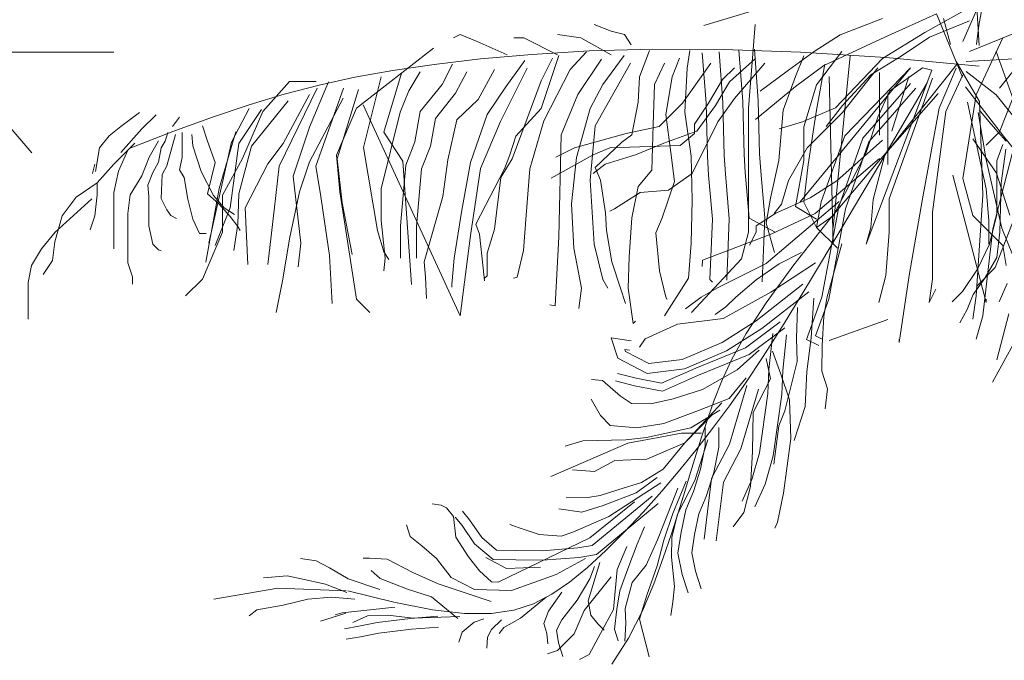
# Model space of a CAD drawing. Units: millimetres. Extents: x 595116 to 630915, y 909473 to 920225.
# Tile 20 of 134: x 629595.85 to 629606.56, y 919164.94 to 919171.91. Entities that reach past the tile are written whole.
import ezdxf

# ---------------------------------------------------------------- set-up
doc = ezdxf.new("R2010")
doc.units = ezdxf.units.MM
doc.layers.add('Dimension', color=3, linetype='Continuous', lineweight=18)
doc.layers.add('L-PLNT', color=85, linetype='Continuous', lineweight=13)
doc.styles.get("Standard").update_dxf_attribs({"font": 'arial.ttf'})
doc.dimstyles.new('ISO-25', dxfattribs={"dimtxt": 9, "dimasz": 6, "dimexe": 1.25, "dimexo": 0.625, "dimtad": 1, "dimlunit": 4, "dimtxsty": 'Standard', "dimcen": 2.5, "dimadec": 0, "dimazin": 0, "dimtfac": 1, "dimtmove": 0, "dimatfit": 3, "dimfxl": 1, "dimarcsym": 0})

# ---------------------------------------------------------------- blocks, each defined once
blk = doc.blocks.new('A$C143125F4')
for p, q in [((4.4749, 1.5142), (4.6718, 1.5142)), ((4.5077, 1.4963), (4.5843, 1.4067))]:
    blk.add_line(p, q)
blk = doc.blocks.new('A$C4FB75ABC')
for p, q in [((2.1827, 2.4393), (1.9579, 2.3712)), ((2.7686, 2.4461), (2.755, 2.3712)), ((2.4825, 2.3372), (2.6324, 2.4053)), ((2.7073, 2.4121), (2.5983, 2.3508)), ((2.6324, 2.4053), (2.7073, 2.2214)), ((2.7083, 2.3255), (2.7471, 2.4129)), ((2.7559, 2.3132), (2.7489, 2.4244)), ((1.6891, 2.3546), (1.6405, 2.3741)), ((2.1065, 2.3741), (2.087, 2.1315)), ((2.353, 2.344), (2.4757, 2.3917)), ((2.7277, 2.3849), (2.6119, 2.3372)), ((2.6732, 2.3168), (2.6528, 2.3917)), ((2.755, 2.3712), (2.7482, 2.3168)), ((1.2522, 2.3449), (1.2328, 2.3352)), ((1.3008, 2.3255), (1.2522, 2.3449)), ((1.6017, 2.3352), (1.5337, 2.3449)), ((1.7279, 2.3449), (1.6891, 2.3546)), ((1.7473, 2.3158), (1.7279, 2.3449)), ((2.2781, 2.2963), (2.353, 2.344)), ((2.5983, 2.3508), (2.4757, 2.2759)), ((2.7277, 2.2964), (2.8733, 2.3546)), ((1.3881, 2.2867), (1.3008, 2.3255)), ((1.4367, 2.3352), (1.4075, 2.3352)), ((1.5337, 2.2867), (1.4367, 2.3352)), ((1.6891, 2.2867), (1.6017, 2.3352)), ((2.3054, 2.2555), (2.4825, 2.3372)), ((2.6119, 2.3372), (2.5302, 2.2827)), ((2.8248, 2.3352), (2.7471, 2.1703)), ((1.1746, 2.3061), (0.9513, 2.1315)), ((1.4598, 2.2878), (1.3106, 2.2744)), ((1.6258, 2.2976), (1.4598, 2.2878)), ((1.5376, 2.2844), (1.4866, 2.1313)), ((1.6179, 2.2954), (1.5705, 2.2443)), ((1.8099, 2.3026), (1.6258, 2.2976)), ((1.7274, 2.2844), (1.6654, 2.2006)), ((1.8004, 2.299), (1.7712, 2.2224)), ((2.0136, 2.3019), (1.8099, 2.3026)), ((1.9171, 2.299), (1.9098, 2.248)), ((1.9536, 2.2917), (1.9646, 2.1459)), ((2.0023, 2.2954), (2.0134, 2.1483)), ((2.2382, 2.2942), (2.0136, 2.3019)), ((2.0597, 2.2997), (2.0708, 2.1511)), ((2.1047, 2.3031), (2.1159, 2.1533)), ((2.2032, 2.2419), (2.2781, 2.2963)), ((2.2482, 2.2839), (2.2239, 2.2232)), ((2.4852, 2.2785), (2.2382, 2.2942)), ((2.3575, 2.296), (2.2846, 2.199)), ((2.3818, 2.2839), (2.3332, 1.7863)), ((2.718, 2.2673), (3.0675, 2.2867)), ((2.8054, 2.2964), (2.8539, 2.1606)), ((1.1767, 2.2586), (1.0564, 2.241)), ((1.3106, 2.2744), (1.1767, 2.2586)), ((1.23, 2.2589), (1.1992, 2.2008)), ((1.4391, 2.2699), (1.3844, 2.1933)), ((1.5194, 2.2771), (1.4866, 2.2115)), ((1.6617, 2.2735), (1.5924, 2.1714)), ((1.7456, 2.2626), (1.6435, 2.0802)), ((1.8442, 2.2626), (1.815, 2.2006)), ((1.8879, 2.2771), (1.8661, 2.2224)), ((1.9783, 2.2623), (1.8966, 2.1465)), ((2.1078, 2.2759), (2.0328, 2.2078)), ((2.135, 2.2623), (2.0465, 2.1602)), ((2.2236, 2.1942), (2.3054, 2.2555)), ((2.3089, 2.2596), (2.2846, 2.1261)), ((2.4757, 2.2759), (2.3394, 2.1329)), ((2.5302, 2.2827), (2.4416, 2.2282)), ((2.6937, 2.2623), (2.4825, 1.9967)), ((2.7559, 2.2536), (2.4852, 2.2785)), ((2.6889, 2.2673), (2.7568, 2.1509)), ((1.0564, 2.241), (0.9464, 2.2213)), ((1.0815, 2.2334), (1.0304, 2.062)), ((1.1363, 2.237), (1.1034, 2.1823)), ((1.2713, 2.237), (1.2384, 2.175)), ((1.3515, 2.2443), (1.3041, 2.1568)), ((1.4464, 2.2479), (1.3687, 2.0927)), ((1.5705, 2.2443), (1.4939, 2.0948)), ((1.9098, 2.248), (1.9025, 2.1203)), ((2.0124, 2.2146), (2.0465, 2.2487)), ((2.1214, 2.1806), (2.2032, 2.2419)), ((2.5574, 2.2487), (2.2372, 1.8605)), ((2.462, 2.2487), (2.3599, 2.1193)), ((2.4416, 2.2282), (2.3599, 2.1397)), ((2.3667, 2.0512), (2.5574, 2.2487)), ((2.428, 1.738), (2.6187, 2.2419)), ((2.4668, 2.2354), (2.4668, 2.0533)), ((2.5915, 2.2487), (2.4961, 2.1806)), ((2.6187, 2.2419), (2.5915, 2.2487)), ((2.6889, 2.2479), (2.6404, 2.1315)), ((2.7083, 2.2285), (2.6598, 2.1218)), ((2.718, 2.2382), (2.8054, 2.1703)), ((2.8151, 2.1897), (2.8539, 2.2382)), ((0.7572, 2.2091), (0.6795, 2.1218)), ((0.8429, 2.1986), (0.7422, 2.1723)), ((0.8348, 2.2091), (0.7572, 2.2091)), ((0.8699, 2.2079), (0.8151, 2.0766)), ((0.9464, 2.2213), (0.8429, 2.1986)), ((1.0231, 2.2224), (0.972, 2.0182)), ((1.1992, 2.2008), (1.1362, 2.1221)), ((1.4866, 2.2115), (1.4464, 2.1021)), ((1.6654, 2.2006), (1.6289, 2.1313)), ((1.7712, 2.2224), (1.7675, 2.1495)), ((1.815, 2.2006), (1.8113, 2.0838)), ((1.8661, 2.2224), (1.8478, 2.113)), ((1.9715, 2.1465), (2.0124, 2.2146)), ((2.0328, 2.2078), (1.992, 2.1397)), ((2.2239, 2.2232), (2.1875, 2.1261)), ((2.2846, 2.199), (2.2482, 2.0776)), ((2.3211, 2.2232), (2.3332, 1.7378)), ((2.5572, 2.203), (2.4187, 2.0449)), ((2.6056, 2.2048), (2.4676, 1.9701)), ((2.6209, 2.2188), (2.4948, 1.8695)), ((2.5518, 2.2232), (2.5032, 2.0655)), ((0.7422, 2.1723), (0.6405, 2.1416)), ((0.837, 2.1896), (0.7276, 1.9635)), ((0.8151, 2.1714), (0.7385, 2.0291)), ((0.9137, 2.1896), (0.8334, 1.9635)), ((0.9575, 2.186), (0.8954, 1.9854)), ((1.1034, 2.1823), (1.0779, 2.1203)), ((1.2384, 2.175), (1.18, 2.1021)), ((1.3844, 2.1933), (1.3297, 2.113)), ((1.5924, 2.1714), (1.5449, 2.0547)), ((2.1078, 2.0989), (2.2236, 2.1942)), ((2.5724, 2.1897), (2.4365, 2.0345)), ((2.4961, 2.1806), (2.462, 2.1057)), ((2.6368, 2.1742), (2.4628, 1.9766)), ((2.4911, 2.1747), (2.4911, 1.9684)), ((2.7471, 2.1703), (2.7083, 1.9277)), ((2.7162, 2.1941), (2.8268, 2.0511)), ((2.8054, 2.1703), (2.883, 2.0733)), ((0.6405, 2.1416), (0.5342, 2.1057)), ((0.7531, 2.1531), (0.6473, 2.0218)), ((0.9125, 2.1606), (0.8154, 1.9763)), ((1.2522, 1.53), (0.9707, 2.1412)), ((1.3041, 2.1568), (1.2421, 2.0984)), ((1.7675, 2.1495), (1.7493, 2.0547)), ((1.8966, 2.1465), (1.8285, 2.0784)), ((1.9306, 2.0852), (1.9715, 2.1465)), ((1.9646, 2.1459), (1.9682, 1.9927)), ((2.0465, 2.1602), (1.9988, 2.0921)), ((2.0134, 2.1483), (2.017, 1.9949)), ((2.0708, 2.1511), (2.0745, 1.9975)), ((2.1159, 2.1533), (2.1196, 1.9995)), ((2.7225, 2.1495), (2.753, 2.0047)), ((2.7568, 2.1509), (2.7666, 1.8792)), ((2.8927, 2.1606), (2.7957, 1.7822)), ((2.8539, 2.1606), (2.8151, 2.0636)), ((0.2683, 2.0784), (0.3228, 2.1193)), ((0.3296, 2.0716), (0.3705, 2.1125)), ((0.64, 2.1313), (0.5889, 2.0328)), ((0.6765, 2.1276), (0.6108, 2.0291)), ((0.6795, 2.1218), (0.6213, 1.986)), ((0.9513, 2.1315), (0.8931, 1.9957)), ((1.0779, 2.1203), (1.0231, 1.8978)), ((1.1362, 2.1221), (1.1203, 2.0346)), ((1.3297, 2.113), (1.2822, 1.9744)), ((1.4866, 2.1313), (1.4136, 2.051)), ((1.6289, 2.1313), (1.5887, 1.989)), ((1.8478, 2.113), (1.8624, 2.0036)), ((1.9025, 2.1203), (1.9208, 1.9927)), ((1.992, 2.1397), (1.9375, 2.0648)), ((2.087, 2.1315), (2.087, 1.7725)), ((2.1875, 2.1261), (2.1754, 1.9805)), ((2.3394, 2.1329), (2.244, 2.0921)), ((2.3599, 2.1193), (2.2577, 2.0172)), ((2.2846, 2.1261), (2.2604, 1.9684)), ((2.3599, 2.1397), (2.3122, 2.0784)), ((2.6404, 2.1315), (2.5918, 1.8695)), ((2.6598, 2.1218), (2.6209, 1.8307)), ((2.753, 2.119), (2.7759, 1.9818)), ((2.7555, 2.1274), (2.7844, 2.0931)), ((0.4182, 2.0784), (0.4386, 2.1057)), ((0.5342, 2.1057), (0.4195, 2.0639)), ((1.18, 2.1021), (1.1654, 2.0218)), ((1.2421, 2.0984), (1.2165, 1.9817)), ((1.3687, 2.0927), (1.3105, 1.9569)), ((1.4464, 2.1021), (1.4026, 1.9854)), ((1.4939, 2.0948), (1.4537, 1.9562)), ((1.8113, 2.0838), (1.8077, 1.9526)), ((1.9988, 2.0921), (1.9238, 1.9422)), ((1.9306, 2.058), (1.9306, 2.0852)), ((2.244, 2.0921), (2.1759, 2.0716)), ((2.462, 2.1057), (2.428, 2.0035)), ((2.7844, 2.0931), (2.8104, 2.0628)), ((0.2342, 2.0512), (0.2683, 2.0784)), ((0.2683, 2.0035), (0.3296, 2.0716)), ((0.4195, 2.0639), (0.2927, 2.0154)), ((0.4049, 2.0609), (0.3966, 2.0361)), ((0.427, 2.0554), (0.4021, 1.9643)), ((0.4463, 2.0609), (0.4463, 1.9892)), ((0.4739, 2.0554), (0.4767, 2.0223)), ((0.505, 2.0802), (0.5196, 2.0364)), ((0.6018, 2.0636), (0.5533, 1.8986)), ((0.8151, 2.0766), (0.7677, 1.9343)), ((1.0304, 2.062), (1.0852, 1.9781)), ((1.5449, 2.0547), (1.5376, 1.7593)), ((1.7331, 2.058), (1.5832, 2.0172)), ((1.6435, 2.0802), (1.6289, 1.9234)), ((1.7493, 2.0547), (1.7201, 2.0328)), ((1.8285, 2.0784), (1.7331, 2.058)), ((1.9375, 2.0648), (1.8421, 2.0308)), ((1.8898, 2.024), (1.9306, 2.058)), ((2.2482, 2.0776), (2.2482, 1.9805)), ((2.8151, 2.0636), (2.7763, 2.0248)), ((2.8104, 2.0628), (2.8339, 2.0359)), ((0.207, 2.0172), (0.2342, 2.0512)), ((0.3092, 2.0308), (0.2479, 1.9695)), ((0.3773, 2.0376), (0.3501, 1.9899)), ((0.3966, 2.0361), (0.3855, 2.0168)), ((0.5196, 2.0364), (0.5415, 1.9744)), ((0.5889, 2.0328), (0.5232, 1.741)), ((0.6108, 2.0291), (0.5853, 1.8431)), ((0.7385, 2.0291), (0.6947, 1.9708)), ((1.1203, 2.0346), (1.0939, 1.9669)), ((1.4136, 2.051), (1.3953, 1.9963)), ((1.7201, 2.0328), (1.6435, 1.9598)), ((1.8421, 2.0308), (1.7603, 1.9967)), ((2.2985, 1.8605), (2.3667, 2.0512)), ((2.4756, 2.0387), (2.3438, 1.9217)), ((2.4187, 2.0449), (2.3489, 1.8456)), ((2.4365, 2.0345), (2.3686, 1.8404)), ((2.7378, 2.0428), (2.8064, 1.9437)), ((2.8244, 2.0263), (2.8071, 1.979)), ((2.8268, 2.0511), (2.9214, 1.9326)), ((0.195, 1.9478), (0.207, 2.0172)), ((0.2887, 2.0103), (0.2615, 1.9491)), ((0.3855, 2.0168), (0.3773, 1.9754)), ((0.4767, 2.0223), (0.5015, 1.9478)), ((0.6473, 2.0218), (0.6108, 1.8833)), ((0.972, 2.0182), (1.0122, 1.7775)), ((1.1654, 2.0218), (1.1399, 1.9562)), ((1.5832, 2.0172), (1.5287, 1.9899)), ((1.6377, 1.9967), (1.6854, 2.0172)), ((1.6854, 2.0172), (1.8898, 2.024)), ((1.8624, 2.0036), (1.8734, 1.9197)), ((2.0745, 1.9975), (2.0779, 1.946)), ((2.1196, 1.9995), (2.1229, 1.9495)), ((2.2577, 2.0172), (2.2032, 1.9218)), ((2.428, 2.0035), (2.3871, 1.9218)), ((2.753, 2.0047), (2.7759, 1.898)), ((2.833, 2.0134), (2.8201, 1.9144)), ((0.1865, 1.9422), (0.1934, 1.9695)), ((0.2479, 1.9695), (0.2002, 1.915)), ((0.3501, 1.9899), (0.3296, 1.9354)), ((0.3773, 1.9754), (0.3607, 1.945)), ((0.4463, 1.9892), (0.438, 1.9533)), ((0.5415, 1.9744), (0.5196, 1.8833)), ((0.6213, 1.986), (0.563, 1.8792)), ((0.6947, 1.9708), (0.629, 1.8431)), ((0.8154, 1.9763), (0.7863, 1.8889)), ((0.8931, 1.9957), (0.9028, 1.8889)), ((0.8954, 1.9854), (0.91, 1.8577)), ((1.0852, 1.9781), (1.1107, 1.6207)), ((1.2165, 1.9817), (1.2019, 1.876)), ((1.2822, 1.9744), (1.2567, 1.8358)), ((1.4026, 1.9854), (1.3698, 1.9307)), ((1.3953, 1.9963), (1.3807, 1.9562)), ((1.5151, 1.9286), (1.6377, 1.9967)), ((1.5887, 1.989), (1.5741, 1.8541)), ((1.6718, 1.9695), (1.6377, 1.9422)), ((1.7603, 1.9967), (1.6718, 1.9695)), ((1.9208, 1.9927), (1.9244, 1.865)), ((1.9682, 1.9927), (1.9719, 1.938)), ((2.017, 1.9949), (2.0206, 1.9417)), ((2.1754, 1.9805), (2.1511, 1.8713)), ((2.2482, 1.9805), (2.2239, 1.847)), ((2.4673, 1.986), (2.2802, 1.8264)), ((2.4628, 1.9766), (2.3249, 1.8127)), ((2.4676, 1.9701), (2.3552, 1.7802)), ((2.4825, 1.9967), (2.4484, 1.8673)), ((2.7759, 1.9818), (2.8217, 1.7836)), ((2.8071, 1.979), (2.8071, 1.9015)), ((0.2615, 1.9491), (0.2479, 1.8878)), ((0.3607, 1.945), (0.3469, 1.9091)), ((0.4021, 1.9643), (0.3883, 1.9395)), ((0.438, 1.9533), (0.4518, 1.9312)), ((0.5015, 1.9478), (0.5374, 1.8788)), ((0.7276, 1.9635), (0.713, 1.8358)), ((0.8334, 1.9635), (0.848, 1.876)), ((1.0939, 1.9669), (1.0786, 1.7905)), ((1.1399, 1.9562), (1.1253, 1.7884)), ((1.3105, 1.9569), (1.2814, 1.7628)), ((1.3807, 1.9562), (1.2968, 1.7957)), ((1.4537, 1.9562), (1.4428, 1.8213)), ((1.6435, 1.9598), (1.6581, 1.9234)), ((1.8077, 1.9526), (1.7675, 1.9051)), ((1.9238, 1.9422), (1.8557, 1.8946)), ((2.0206, 1.9417), (2.0317, 1.8114)), ((2.0779, 1.946), (2.0893, 1.8127)), ((2.1229, 1.9495), (2.1345, 1.8136)), ((2.2604, 1.9684), (2.2482, 1.8591)), ((2.8064, 1.9437), (2.8446, 1.8217)), ((0.2002, 1.915), (0.1389, 1.8742)), ((0.2002, 1.915), (0.2002, 1.881)), ((0.3296, 1.9354), (0.2956, 1.881)), ((0.3883, 1.9395), (0.3855, 1.8705)), ((0.4518, 1.9312), (0.4629, 1.8677)), ((0.7677, 1.9343), (0.7896, 1.741)), ((1.3698, 1.9307), (1.3515, 1.7811)), ((1.6289, 1.9234), (1.6398, 1.7374)), ((1.6581, 1.9234), (1.6727, 1.8285)), ((1.8734, 1.9197), (1.8369, 1.814)), ((1.9719, 1.938), (1.9828, 1.8103)), ((2.2032, 1.9218), (2.1827, 1.8537)), ((2.3438, 1.9217), (2.2657, 1.8718)), ((2.3871, 1.9218), (2.3326, 1.8197)), ((2.6792, 1.9375), (2.7763, 1.5688)), ((2.7083, 1.9277), (2.7374, 1.821)), ((2.8201, 1.9144), (2.8158, 1.7724)), ((0.2479, 1.8878), (0.2479, 1.8061)), ((0.3469, 1.9091), (0.3497, 1.876)), ((0.5533, 1.8986), (0.5339, 1.7919)), ((0.7863, 1.8889), (0.7572, 1.7531)), ((0.9028, 1.8889), (0.9513, 1.5785)), ((1.0231, 1.8978), (1.0231, 1.8067)), ((1.7739, 1.8878), (1.699, 1.8401)), ((1.7675, 1.9051), (1.7493, 1.814)), ((1.8557, 1.8946), (1.7739, 1.8878)), ((2.7759, 1.898), (2.7836, 1.8065)), ((2.8071, 1.9015), (2.8071, 1.8241)), ((0.1844, 1.8695), (0.0777, 1.7725)), ((0.1389, 1.8742), (0.098, 1.8197)), ((0.2002, 1.881), (0.1934, 1.8197)), ((0.2956, 1.881), (0.2887, 1.8265)), ((0.3497, 1.876), (0.3497, 1.8512)), ((0.3855, 1.8705), (0.4021, 1.8374)), ((0.4629, 1.8677), (0.4767, 1.8098)), ((0.5196, 1.8833), (0.5524, 1.8541)), ((0.5374, 1.8788), (0.5678, 1.8429)), ((0.563, 1.8792), (0.563, 1.7725)), ((0.6108, 1.8833), (0.6072, 1.7957)), ((0.848, 1.876), (0.8735, 1.7045)), ((0.91, 1.8577), (0.9392, 1.7082)), ((1.2019, 1.876), (1.1472, 1.6863)), ((1.9244, 1.865), (1.9208, 1.741)), ((2.3505, 1.8613), (2.1386, 1.6813)), ((2.1511, 1.8713), (2.1389, 1.7985)), ((2.2657, 1.8718), (2.167, 1.8279)), ((2.2482, 1.8591), (2.2846, 1.7863)), ((2.2849, 1.7856), (2.2985, 1.8605)), ((2.4484, 1.8673), (2.4416, 1.7856)), ((2.4948, 1.8695), (2.4948, 1.7725)), ((2.5918, 1.8695), (2.553, 1.6464)), ((2.7666, 1.8792), (2.7471, 1.5882)), ((0.2887, 1.8265), (0.2887, 1.7516)), ((0.3497, 1.8512), (0.3497, 1.7904)), ((0.4021, 1.8374), (0.4132, 1.8208)), ((0.5853, 1.8431), (0.5415, 1.7337)), ((0.5524, 1.8541), (0.5853, 1.8176)), ((0.5678, 1.8429), (0.5982, 1.8236)), ((0.629, 1.8431), (0.6363, 1.679)), ((0.713, 1.8358), (0.6984, 1.7118)), ((1.2567, 1.8358), (1.2348, 1.6973)), ((1.5741, 1.8541), (1.5814, 1.7264)), ((1.6727, 1.8285), (1.6763, 1.7775)), ((1.699, 1.8401), (1.6854, 1.8333)), ((2.167, 1.8279), (2.1099, 1.791)), ((2.2802, 1.8264), (2.1549, 1.7678)), ((2.1827, 1.8537), (2.1623, 1.8265)), ((2.2239, 1.847), (2.2846, 1.8106)), ((2.3489, 1.8456), (2.3004, 1.5838)), ((2.3686, 1.8404), (2.32, 1.5785)), ((2.6209, 1.8307), (2.6209, 1.6367)), ((2.8708, 1.8469), (2.8027, 1.6699)), ((0.098, 1.8197), (0.0775, 1.7448)), ((0.1934, 1.8197), (0.1797, 1.7788)), ((0.2479, 1.8061), (0.2479, 1.7448)), ((0.4132, 1.8208), (0.4297, 1.8125)), ((0.4767, 1.8098), (0.496, 1.7684)), ((0.5853, 1.8176), (0.6072, 1.7884)), ((1.0231, 1.8067), (1.0341, 1.6973)), ((1.4428, 1.8213), (1.4355, 1.7191)), ((1.7493, 1.814), (1.742, 1.7009)), ((1.8369, 1.814), (1.8186, 1.7702)), ((1.9828, 1.8103), (1.9755, 1.6352)), ((2.0317, 1.8114), (2.0243, 1.6332)), ((2.0893, 1.8127), (2.1647, 1.7725)), ((2.1345, 1.8136), (2.1268, 1.6289)), ((2.1389, 1.7985), (2.1632, 1.7135)), ((2.3249, 1.8127), (2.2184, 1.678)), ((2.3326, 1.8197), (2.2849, 1.7856)), ((2.7374, 1.821), (2.8248, 1.7337)), ((2.7836, 1.8065), (2.7836, 1.7379)), ((2.8071, 1.8241), (2.7856, 1.738)), ((0.0777, 1.7725), (0.0388, 1.724)), ((0.3497, 1.7904), (0.3607, 1.738)), ((0.563, 1.7725), (0.5048, 1.6367)), ((0.5339, 1.7919), (0.5145, 1.6852)), ((0.6072, 1.7957), (0.5962, 1.7191)), ((0.6072, 1.7884), (0.6144, 1.7775)), ((1.0122, 1.7775), (1.0304, 1.7155)), ((1.0786, 1.7905), (1.0786, 1.6973)), ((1.1253, 1.7884), (1.1253, 1.7665)), ((1.2968, 1.7957), (1.3078, 1.7665)), ((1.3515, 1.7811), (1.3297, 1.7118)), ((1.6763, 1.7775), (1.6909, 1.6863)), ((1.8186, 1.7702), (1.8296, 1.6608)), ((2.087, 1.7725), (2.0676, 1.6949)), ((2.1096, 1.7722), (2.0903, 1.7347)), ((2.1099, 1.791), (2.1096, 1.7722)), ((2.3552, 1.7802), (2.2641, 1.6283)), ((2.2846, 1.7863), (2.3453, 1.7256)), ((2.4416, 1.7856), (2.428, 1.738)), ((2.4948, 1.7725), (2.485, 1.6464)), ((2.7957, 1.7822), (2.7666, 1.53)), ((2.8158, 1.7724), (2.8071, 1.6993)), ((2.8217, 1.7836), (2.8522, 1.7074)), ((0.0775, 1.7448), (0.0707, 1.6903)), ((0.2479, 1.7448), (0.2479, 1.7243)), ((0.2887, 1.7516), (0.2887, 1.6835)), ((0.496, 1.7684), (0.5153, 1.7684)), ((0.7572, 1.7531), (0.7377, 1.6367)), ((0.7896, 1.741), (0.7823, 1.6717)), ((1.1253, 1.7665), (1.1253, 1.7301)), ((1.2814, 1.7628), (1.2522, 1.53)), ((1.3078, 1.7665), (1.3187, 1.6681)), ((1.5376, 1.7593), (1.5267, 1.5587)), ((1.9208, 1.741), (1.9135, 1.6389)), ((2.1549, 1.7678), (1.9538, 1.6913)), ((0.0388, 1.724), (0.0097, 1.6755)), ((0.3607, 1.738), (0.3773, 1.7214)), ((0.3773, 1.7214), (0.3855, 1.7187)), ((1.0304, 1.7155), (1.045, 1.6936)), ((1.1253, 1.7301), (1.1253, 1.6973)), ((1.4355, 1.7191), (1.4172, 1.6425)), ((1.5814, 1.7264), (1.6033, 1.6097)), ((1.6398, 1.7374), (1.6654, 1.6352)), ((2.2409, 1.7138), (2.1763, 1.6807)), ((2.3582, 1.7386), (2.3145, 1.5808)), ((2.7856, 1.738), (2.7512, 1.6648)), ((2.8248, 1.7337), (2.8345, 1.6755)), ((0.0707, 1.6903), (0.0435, 1.6494)), ((0.6984, 1.7118), (0.6947, 1.679)), ((0.8735, 1.7045), (0.8808, 1.566)), ((1.0341, 1.6973), (1.0304, 1.6608)), ((1.1472, 1.6863), (1.1509, 1.6425)), ((1.2348, 1.6973), (1.2275, 1.6207)), ((1.3297, 1.7118), (1.3297, 1.6462)), ((1.6909, 1.6863), (1.7164, 1.6097)), ((1.742, 1.7009), (1.7383, 1.6097)), ((2.0676, 1.6949), (1.922, 1.5397)), ((1.9538, 1.6913), (1.9536, 1.6725)), ((2.8071, 1.6993), (2.7727, 1.639)), ((0.0097, 1.6755), (0, 1.627)), ((0.2887, 1.6835), (0.3024, 1.6426)), ((1.3187, 1.6681), (1.3224, 1.6316)), ((1.8296, 1.6608), (1.8478, 1.5842)), ((2.1386, 1.6813), (1.998, 1.6115)), ((2.1763, 1.6807), (2.1096, 1.6345)), ((2.2184, 1.678), (2.1385, 1.568)), ((2.2819, 1.6831), (2.1525, 1.5981)), ((2.7512, 1.6648), (2.7081, 1.6003)), ((2.8027, 1.6699), (2.7482, 1.6154)), ((0, 1.627), (0, 1.5494)), ((0.3024, 1.6426), (0.3024, 1.6222)), ((0.5048, 1.6367), (0.4562, 1.5882)), ((0.7377, 1.6367), (0.7183, 1.5397)), ((1.1509, 1.6425), (1.1545, 1.5805)), ((1.3297, 1.6462), (1.3224, 1.6389)), ((1.4172, 1.6425), (1.4063, 1.6389)), ((1.6654, 1.6352), (1.68, 1.6097)), ((1.9135, 1.6389), (1.8444, 1.53)), ((1.9755, 1.6352), (1.9828, 1.628)), ((2.1096, 1.6345), (2.0504, 1.5844)), ((2.2641, 1.6283), (2.1904, 1.5079)), ((2.485, 1.6464), (2.4656, 1.5688)), ((2.553, 1.6464), (2.5239, 1.4523)), ((2.6209, 1.6367), (2.6112, 1.5688)), ((2.7727, 1.639), (2.7383, 1.5917)), ((1.2275, 1.6207), (1.2275, 1.6134)), ((1.6033, 1.6097), (1.596, 1.5514)), ((1.7164, 1.6097), (1.731, 1.566)), ((1.7383, 1.6097), (1.7529, 1.5076)), ((1.998, 1.6115), (1.9504, 1.5839)), ((2.1525, 1.5981), (2.0137, 1.5227)), ((2.2452, 1.6213), (2.1098, 1.5157)), ((2.2623, 1.5995), (2.1258, 1.493)), ((2.6112, 1.5688), (2.6307, 1.6076)), ((2.7081, 1.6003), (2.678, 1.5702)), ((2.8369, 1.6236), (2.8141, 1.5702)), ((0.9513, 1.5785), (0.9901, 1.5397)), ((1.8478, 1.5842), (1.8515, 1.5769)), ((1.9504, 1.5839), (1.9047, 1.5506)), ((2.0504, 1.5844), (2.0217, 1.5565)), ((2.3004, 1.5838), (2.256, 1.4617)), ((2.2767, 1.5813), (2.2695, 1.4664)), ((2.32, 1.5785), (2.2812, 1.4717)), ((2.3145, 1.5808), (2.3062, 1.5281)), ((2.7383, 1.5917), (2.721, 1.5486)), ((2.7471, 1.5882), (2.7374, 1.5203)), ((2.7763, 1.5688), (2.7763, 1.5785)), ((0, 1.5494), (0, 1.5203)), ((1.5267, 1.5587), (1.5121, 1.5623)), ((2.0217, 1.5565), (1.9912, 1.5343)), ((2.1385, 1.568), (2.0803, 1.4783)), ((2.2292, 1.5537), (2.2261, 1.4651)), ((2.721, 1.5486), (2.6995, 1.5099)), ((2.9148, 1.5573), (2.7942, 1.3378)), ((1.7529, 1.5076), (1.7602, 1.5149)), ((2.0137, 1.5227), (1.8814, 1.5056)), ((2.1098, 1.5157), (2.0109, 1.453)), ((2.1796, 1.5129), (2.0785, 1.437)), ((2.3062, 1.5281), (2.3013, 1.4452)), ((2.4911, 1.5193), (2.3211, 1.4586)), ((2.7666, 1.53), (2.7471, 1.462)), ((2.8416, 1.5357), (2.8071, 1.4023)), ((1.8814, 1.5056), (1.7884, 1.4636)), ((2.1258, 1.493), (2.0238, 1.4284)), ((2.1927, 1.4954), (2.0894, 1.4177)), ((2.1904, 1.5079), (2.1298, 1.4122)), ((1.7084, 1.4073), (1.6895, 1.4666)), ((1.6895, 1.4666), (1.747, 1.4576)), ((1.7884, 1.4636), (1.7711, 1.4393)), ((2.0803, 1.4783), (2.039, 1.4043)), ((2.1578, 1.4791), (2.1468, 1.3743)), ((2.1979, 1.4749), (2.187, 1.3714)), ((2.2261, 1.4651), (2.2289, 1.3972)), ((2.256, 1.4617), (2.2916, 1.4439)), ((2.2695, 1.4664), (2.2568, 1.3685)), ((2.2812, 1.4717), (2.3006, 1.462)), ((2.5239, 1.4523), (2.5239, 1.462)), ((1.7313, 1.4266), (1.7295, 1.4323)), ((1.7295, 1.4323), (1.7427, 1.4302)), ((2.0109, 1.453), (1.8951, 1.4036)), ((2.0238, 1.4284), (1.9024, 1.3766)), ((2.0785, 1.437), (1.9344, 1.3786)), ((2.1181, 1.4308), (2.055, 1.3732)), ((2.1569, 1.4277), (2.1816, 1.3609)), ((2.3013, 1.4452), (2.3002, 1.3698)), ((1.7936, 1.3632), (1.7084, 1.4073)), ((1.7987, 1.3918), (1.7313, 1.4266)), ((1.8951, 1.4036), (1.7987, 1.3918)), ((2.0894, 1.4177), (1.9429, 1.3584)), ((2.039, 1.4043), (2.0098, 1.3416)), ((2.1298, 1.4122), (2.0784, 1.3347)), ((2.1385, 1.406), (2.1509, 1.3473)), ((1.9024, 1.3766), (1.7936, 1.3632)), ((1.9344, 1.3786), (1.8357, 1.3347)), ((2.055, 1.3732), (1.9542, 1.3161)), ((2.1468, 1.3743), (2.1439, 1.3053)), ((2.187, 1.3714), (2.1842, 1.3016)), ((2.2289, 1.3972), (2.1929, 1.2544)), ((2.3002, 1.3698), (2.3165, 1.3187)), ((1.6641, 1.3427), (1.6321, 1.345)), ((1.7163, 1.2967), (1.6641, 1.3427)), ((1.7575, 1.3275), (1.7024, 1.3416)), ((1.7623, 1.3489), (1.7078, 1.3628)), ((1.8357, 1.3347), (1.7623, 1.3489)), ((1.9429, 1.3584), (1.8383, 1.3119)), ((2.0098, 1.3416), (1.9878, 1.2857)), ((2.0811, 1.3502), (2.0312, 1.2905)), ((2.1509, 1.3473), (2.1005, 1.25)), ((2.1816, 1.3609), (2.2062, 1.287)), ((2.2568, 1.3685), (2.2516, 1.2668)), ((1.8383, 1.3119), (1.7575, 1.3275)), ((1.9542, 1.3161), (1.869, 1.289)), ((2.0784, 1.3347), (2.0319, 1.2687)), ((2.0829, 1.3276), (2.0324, 1.158)), ((2.1165, 1.3176), (2.065, 1.1449)), ((2.3165, 1.3187), (2.31, 1.2603)), ((1.6589, 1.2409), (1.6313, 1.2885)), ((1.7481, 1.2755), (1.7163, 1.2967)), ((1.869, 1.289), (1.8046, 1.2748)), ((2.0312, 1.2905), (1.9421, 1.2559)), ((1.9878, 1.2857), (1.9691, 1.2327)), ((2.1439, 1.3053), (2.1195, 1.1332)), ((2.1842, 1.3016), (2.1591, 1.1247)), ((2.2062, 1.287), (2.2097, 1.1745)), ((1.8046, 1.2748), (1.7481, 1.2755)), ((1.9421, 1.2559), (1.8416, 1.2177)), ((2.0103, 1.2776), (1.903, 1.1622)), ((2.0043, 1.257), (1.9206, 1.2053)), ((2.0319, 1.2687), (1.9864, 1.2075)), ((2.2516, 1.2668), (2.22, 1.1691)), ((1.6868, 1.2123), (1.6589, 1.2409)), ((1.9834, 1.244), (1.903, 1.1622)), ((1.9691, 1.2327), (1.952, 1.1808)), ((2.1005, 1.25), (2.0989, 1.1369)), ((2.1929, 1.2544), (2.1754, 1.2112)), ((1.7641, 1.2056), (1.6868, 1.2123)), ((1.8416, 1.2177), (1.7641, 1.2056)), ((1.9206, 1.2053), (1.792, 1.1769)), ((1.9864, 1.2075), (1.9386, 1.1458)), ((1.9621, 1.2066), (1.9614, 1.1536)), ((2.0017, 1.2061), (2.001, 1.1495)), ((2.1754, 1.2112), (2.1606, 1.1002)), ((1.7315, 1.1702), (1.607, 1.1681)), ((1.792, 1.1769), (1.7315, 1.1702)), ((1.7376, 1.1613), (1.8929, 1.1904)), ((1.8929, 1.1904), (1.9511, 1.1904)), ((1.9692, 1.1707), (1.9317, 1.0524)), ((1.952, 1.1808), (1.9358, 1.129)), ((2.2097, 1.1745), (2.1886, 1.0162)), ((1.5143, 1.0642), (1.7376, 1.1613)), ((1.607, 1.1681), (1.5558, 1.1518)), ((1.903, 1.1622), (1.793, 1.1147)), ((1.903, 1.1622), (1.8397, 1.0857)), ((1.9386, 1.1458), (1.8882, 1.0835)), ((1.9614, 1.1536), (1.9482, 1.0859)), ((2.0324, 1.158), (1.9806, 1.0581)), ((2.001, 1.1495), (1.9867, 1.0762)), ((2.065, 1.1449), (2.0146, 1.0475)), ((1.793, 1.1147), (1.7005, 1.1103)), ((1.9358, 1.129), (1.9198, 1.076)), ((2.0989, 1.1369), (2.0937, 1.0351)), ((2.1195, 1.1332), (2.0972, 1.056)), ((2.1591, 1.1247), (2.1353, 1.0421)), ((1.7005, 1.1103), (1.6416, 1.079)), ((1.8397, 1.0857), (1.7769, 1.047)), ((1.9482, 1.0859), (1.9278, 1.0204)), ((1.6416, 1.079), (1.5775, 1.0837)), ((1.8224, 1.0615), (1.7614, 1.017)), ((1.8882, 1.0835), (1.8359, 1.0215)), ((1.9198, 1.076), (1.903, 1.0206)), ((1.9806, 1.0581), (1.9586, 0.8825)), ((1.9867, 1.0762), (1.965, 1.0067)), ((2.0972, 1.056), (2.0692, 0.9929)), ((1.8335, 1.0462), (1.6831, 0.9483)), ((1.7769, 1.047), (1.7087, 1.0253)), ((1.8823, 1.0305), (1.8549, 0.9592)), ((1.9071, 1.0509), (1.8681, 0.9571)), ((1.9317, 1.0524), (1.8813, 0.9551)), ((2.0146, 1.0475), (2.004, 0.9628)), ((2.0937, 1.0351), (2.0738, 0.96)), ((2.1353, 1.0421), (2.1061, 0.9765)), ((1.6216, 1.0039), (1.5594, 1.0028)), ((1.6576, 1.009), (1.6216, 1.0039)), ((1.8084, 1.007), (1.6348, 0.8642)), ((1.7087, 1.0253), (1.6576, 1.009)), ((1.7614, 1.017), (1.6666, 0.9806)), ((1.8359, 1.0215), (1.7823, 0.9612)), ((1.903, 1.0206), (1.8847, 0.9618)), ((1.9278, 1.0204), (1.9055, 0.9679)), ((1.965, 1.0067), (1.9435, 0.9561)), ((2.1886, 1.0162), (2.171, 0.9318)), ((1.1969, 0.9814), (1.1705, 0.9855)), ((1.2119, 0.9737), (1.1969, 0.9814)), ((1.2323, 0.9489), (1.2119, 0.9737)), ((1.6041, 0.9607), (1.5382, 0.9711)), ((1.6666, 0.9806), (1.6041, 0.9607)), ((1.7573, 0.9907), (1.6276, 0.8869)), ((1.8259, 0.9857), (1.6466, 0.8382)), ((1.239, 0.8884), (1.2323, 0.9489)), ((1.2572, 0.9222), (1.2376, 0.9461)), ((1.2793, 0.9388), (1.2589, 0.9636)), ((1.6831, 0.9483), (1.5787, 0.9026)), ((1.7823, 0.9612), (1.7281, 0.9036)), ((1.8549, 0.9592), (1.8236, 0.8804)), ((1.8681, 0.9571), (1.8425, 0.8802)), ((1.8847, 0.9618), (1.8642, 0.8983)), ((1.8813, 0.9551), (1.8652, 0.8874)), ((1.9055, 0.9679), (1.8924, 0.9029)), ((1.9435, 0.9561), (1.9314, 0.8959)), ((2.004, 0.9628), (1.9934, 0.8781)), ((2.0738, 0.96), (2.043, 0.9189)), ((1.107, 0.8902), (1.0961, 0.9243)), ((1.2938, 0.8688), (1.2572, 0.9222)), ((1.3144, 0.8874), (1.2793, 0.9388)), ((1.4036, 0.922), (1.3961, 0.9259)), ((1.4317, 0.9122), (1.4036, 0.922)), ((1.7864, 0.9186), (1.765, 0.868)), ((2.171, 0.9318), (2.164, 0.9142)), ((1.1405, 0.8634), (1.107, 0.8902)), ((1.2759, 0.8314), (1.239, 0.8884)), ((1.3573, 0.851), (1.3144, 0.8874)), ((1.6276, 0.8869), (1.3617, 0.7585)), ((1.4805, 0.8964), (1.4317, 0.9122)), ((1.5446, 0.8918), (1.4805, 0.8964)), ((1.5787, 0.9026), (1.5446, 0.8918)), ((1.7281, 0.9036), (1.6739, 0.8498)), ((1.8642, 0.8983), (1.8405, 0.829)), ((1.8652, 0.8874), (1.8644, 0.8308)), ((1.8924, 0.9029), (1.8829, 0.8424)), ((1.9314, 0.8959), (1.9231, 0.8432)), ((1.1834, 0.827), (1.1405, 0.8634)), ((1.347, 0.8236), (1.2938, 0.8688)), ((1.5932, 0.8572), (1.4893, 0.8492)), ((1.6348, 0.8642), (1.5932, 0.8572)), ((1.7347, 0.8614), (1.7065, 0.7946)), ((1.765, 0.868), (1.7376, 0.7967)), ((1.8236, 0.8804), (1.7906, 0.8073)), ((1.8425, 0.8802), (1.8226, 0.805)), ((0.9891, 0.8277), (0.9703, 0.828)), ((1.04, 0.8252), (0.9891, 0.8277)), ((1.3074, 0.7913), (1.2759, 0.8314)), ((1.3863, 0.7981), (1.3265, 0.8298)), ((1.4139, 0.8502), (1.3573, 0.851)), ((1.4893, 0.8492), (1.4139, 0.8502)), ((1.5965, 0.8298), (1.4902, 0.8216)), ((1.6466, 0.8382), (1.5965, 0.8298)), ((1.6739, 0.8498), (1.6204, 0.8011)), ((1.8405, 0.829), (1.8129, 0.7535)), ((1.8644, 0.8308), (1.8727, 0.7459)), ((1.8829, 0.8424), (1.8952, 0.7804)), ((1.9231, 0.8432), (1.9337, 0.7903)), ((0.8346, 0.8198), (0.7888, 0.827)), ((0.8736, 0.7996), (0.8346, 0.8198)), ((0.9273, 0.7678), (0.8736, 0.7996)), ((1.1149, 0.7864), (1.04, 0.8252)), ((1.226, 0.7717), (1.1834, 0.827)), ((1.4135, 0.8227), (1.347, 0.8236)), ((1.4848, 0.8016), (1.3863, 0.7981)), ((1.4902, 0.8216), (1.4135, 0.8227)), ((1.6154, 0.8267), (1.5299, 0.7807)), ((1.6204, 0.8011), (1.5682, 0.7585)), ((1.6567, 0.8148), (1.6231, 0.704)), ((1.6415, 0.8037), (1.6278, 0.7681)), ((1.7906, 0.8073), (1.7502, 0.757)), ((1.8226, 0.805), (1.7931, 0.7206)), ((0.7503, 0.7767), (0.6814, 0.7711)), ((0.7912, 0.768), (0.7503, 0.7767)), ((1.0204, 0.7689), (0.9943, 0.7918)), ((1.188, 0.7534), (1.1149, 0.7864)), ((1.2935, 0.7368), (1.226, 0.7717)), ((1.3428, 0.7588), (1.3074, 0.7913)), ((1.5299, 0.7807), (1.4009, 0.7335)), ((1.6891, 0.7732), (1.6114, 0.6762)), ((1.7065, 0.7946), (1.696, 0.6785)), ((1.7376, 0.7967), (1.7141, 0.733)), ((1.8952, 0.7804), (1.9122, 0.7271)), ((1.9337, 0.7903), (1.9499, 0.7392)), ((0.8615, 0.7523), (0.7912, 0.768)), ((0.9235, 0.7285), (0.8615, 0.7523)), ((1.0187, 0.737), (0.9273, 0.7678)), ((1.0992, 0.7376), (1.0204, 0.7689)), ((1.342, 0.7022), (1.188, 0.7534)), ((1.3617, 0.7585), (1.3428, 0.7588)), ((1.5682, 0.7585), (1.5172, 0.7231)), ((1.6278, 0.7681), (1.5911, 0.7064)), ((1.7502, 0.757), (1.7303, 0.6818)), ((1.8129, 0.7535), (1.7799, 0.6746)), ((1.8727, 0.7459), (1.8683, 0.7007)), ((0.7236, 0.7411), (0.5379, 0.7092)), ((0.9219, 0.7334), (0.7236, 0.7411)), ((0.879, 0.7143), (0.8101, 0.7087)), ((0.9462, 0.7085), (0.879, 0.7143)), ((1.0599, 0.6997), (0.9265, 0.7333)), ((1.1687, 0.7159), (1.0992, 0.7376)), ((1.2451, 0.6526), (1.1687, 0.7159)), ((1.4009, 0.7335), (1.2935, 0.7368)), ((1.5006, 0.7151), (1.4262, 0.6539)), ((1.5172, 0.7231), (1.4647, 0.6957)), ((1.5461, 0.7296), (1.5076, 0.6736)), ((1.7141, 0.733), (1.7058, 0.6803)), ((1.7931, 0.7206), (1.7714, 0.6511)), ((0.7393, 0.6917), (0.6621, 0.678)), ((0.8101, 0.7087), (0.7393, 0.6917)), ((1.0623, 0.6856), (0.9095, 0.6697)), ((1.1712, 0.6779), (1.0599, 0.6997)), ((1.4647, 0.6957), (1.4072, 0.6768)), ((1.5911, 0.7064), (1.5469, 0.6485)), ((1.6231, 0.704), (1.6301, 0.6625)), ((1.8683, 0.7007), (1.8621, 0.6612)), ((0.6621, 0.678), (0.6405, 0.6602)), ((0.9209, 0.6684), (0.8811, 0.6557)), ((0.9095, 0.6697), (0.8898, 0.6634)), ((0.9832, 0.6605), (0.9403, 0.6414)), ((1.0423, 0.6629), (0.9832, 0.6605)), ((1.1159, 0.6537), (1.0423, 0.6629)), ((1.1867, 0.6591), (1.1074, 0.6526)), ((1.2504, 0.6584), (1.1159, 0.6537)), ((1.2639, 0.6673), (1.1712, 0.6779)), ((1.3414, 0.6671), (1.2639, 0.6673)), ((1.4072, 0.6768), (1.3414, 0.6671)), ((1.5076, 0.6736), (1.4939, 0.6379)), ((1.6114, 0.6762), (1.5823, 0.6082)), ((1.6301, 0.6625), (1.6505, 0.6377)), ((1.696, 0.6785), (1.6713, 0.6328)), ((1.7058, 0.6803), (1.6993, 0.6219)), ((1.7303, 0.6818), (1.7316, 0.6384)), ((1.7799, 0.6746), (1.74, 0.5958)), ((0.8811, 0.6557), (0.847, 0.6449)), ((0.9581, 0.6302), (0.9165, 0.6232)), ((1.011, 0.6408), (0.9581, 0.6302)), ((1.1074, 0.6526), (1.011, 0.6408)), ((1.1893, 0.628), (1.1106, 0.6216)), ((1.2921, 0.6426), (1.2578, 0.6129)), ((1.3206, 0.6516), (1.2921, 0.6426)), ((1.3714, 0.649), (1.3428, 0.6211)), ((1.4262, 0.6539), (1.3787, 0.6263)), ((1.4939, 0.6379), (1.5029, 0.6095)), ((1.5469, 0.6485), (1.5314, 0.6186)), ((1.6713, 0.6328), (1.6256, 0.5484)), ((1.6505, 0.6377), (1.6691, 0.6186)), ((1.7316, 0.6384), (1.729, 0.5876)), ((1.7714, 0.6511), (1.8, 0.5413)), ((0.9632, 0.5994), (0.9216, 0.5925)), ((1.016, 0.61), (0.9632, 0.5994)), ((1.1106, 0.6216), (1.016, 0.61)), ((1.2578, 0.6129), (1.2479, 0.5847)), ((1.3428, 0.6211), (1.3311, 0.5987)), ((1.3787, 0.6263), (1.3652, 0.6095)), ((1.5029, 0.6095), (1.5063, 0.5793)), ((1.5314, 0.6186), (1.5365, 0.5827)), ((1.5823, 0.6082), (1.5337, 0.5597)), ((1.6993, 0.6219), (1.7101, 0.5878)), ((1.3311, 0.5987), (1.3288, 0.5666)), ((1.5365, 0.5827), (1.5492, 0.5429)), ((1.74, 0.5958), (1.6917, 0.5207)), ((1.5337, 0.5597), (1.5046, 0.55)), ((1.6256, 0.5484), (1.5974, 0.5343))]:
    blk.add_line(p, q)
blk = doc.blocks.new('*D216')
at = {"layer": 'Defpoints', "color": 0, "transparency": 16777216}
for p in [(629743.541, 919411.928), (629505.041, 919411.828), (629743.541, 918832.378)]:
    blk.add_point(p, dxfattribs=at)
at = {"layer": 'Dimension', "color": 0, "lineweight": -2, "transparency": 16777216}
for p, q in [((629743.541, 919411.303), (629743.541, 918831.128)), ((629505.041, 919411.203), (629505.041, 918831.128)), ((629511.041, 918832.378), (629737.541, 918832.378))]:
    blk.add_line(p, q, dxfattribs=at)
at = {"layer": 'Dimension', "color": 0, "transparency": 16777216}
for points in [[(629511.041, 918833.378), (629511.041, 918831.378), (629505.041, 918832.378)], [(629737.541, 918833.378), (629737.541, 918831.378), (629743.541, 918832.378)]]:
    blk.add_solid(points, dxfattribs=at)
at = {"layer": 'Dimension', "color": 0, "transparency": 16777216, "insert": (629624.291, 918837.656), "char_height": 9, "attachment_point": 5}
blk.add_mtext('19\'-10 1/2"', dxfattribs=at)

msp = doc.modelspace()

# ---------------------------------------------------------------- block references
at = {"layer": 'L-PLNT'}
for name, p, xscale, yscale, zscale in [('A$C143125F4', (629549.214, 919156.111), 10.20167662382051, 10.20167662382051, 10.20167662382051), ('A$C4FB75ABC', (629595.944, 919162.946), 3.753413438031968, 3.753413438031968, 3.753413438031968)]:
    msp.add_blockref(name, p, dxfattribs=dict(at, xscale=xscale, yscale=yscale, zscale=zscale))

# ---------------------------------------------------------------- dimensions: what is measured, and where the dimension line sits
at = {"layer": 'Dimension'}
dim = msp.add_linear_dim(base=(629743.541, 918832.378), p1=(629505.041, 919411.828), p2=(629743.541, 919411.928), dimstyle='ISO-25', override={"dimdec": 1, "dimlfac": 1, "dimrnd": 0, "dimzin": 1, "dimdsep": 46, "dimlunit": 4, "dimfrac": 2}, dxfattribs=at)
dim.commit()
dim.dimension.update_dxf_attribs({"geometry": '*D216', "text_midpoint": (629624.291, 918837.656)})

doc.saveas('drawing.dxf')
